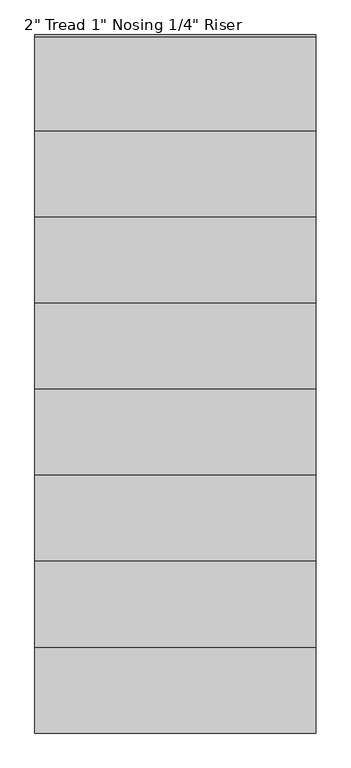
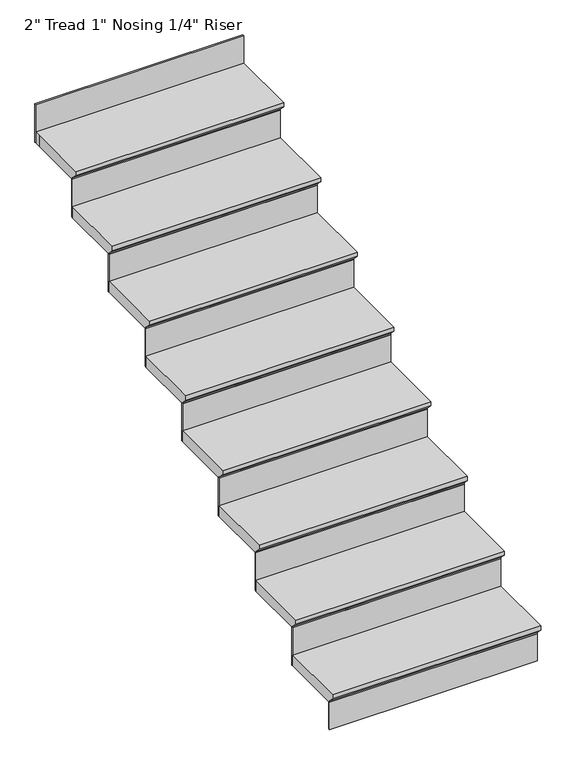
"""IFC4 building model written with IfcOpenShell, lengths in millimetres: stair flight geometry."""

from ifc_helpers import new_model, si_unit, origin, place, context, project, spatial, faceted_brep, source, transform, mapped, element, save


def stair_flight_342035e6(model_context):
    return source(origin(), model_context, "Body", "Brep", [
        faceted_brep([(-11728.968339, 6177.243496, 3968.75), (-11728.968339, 6177.243496, 3987.8), (-12643.368339, 6177.243496, 3987.8), (-12643.368339, 6177.243496, 3968.75), (-11728.968339, 6202.643496, 3943.35), (-12643.368339, 6202.643496, 3943.35), (-11728.968339, 6482.043496, 3987.8), (-12643.368339, 6482.043496, 3987.8), (-12643.368339, 6202.643496, 3937.0), (-12643.368339, 6482.043496, 3937.0), (-11728.968339, 6482.043496, 3937.0), (-11728.968339, 6202.643496, 3937.0)], [[[0, 1, 2, 3]], [[4, 0, 3, 5]], [[2, 1, 6, 7]], [[8, 9, 10, 11]], [[2, 7, 9, 8, 5, 3]], [[8, 11, 4, 5]], [[6, 1, 0, 4, 11, 10]], [[7, 6, 10, 9]]]),
        faceted_brep([(-11728.968339, 6202.643496, 3937.0), (-11728.968339, 6202.643496, 3810.0), (-11728.968339, 6208.993496, 3810.0), (-11728.968339, 6208.993496, 3937.0), (-12643.368339, 6202.643496, 3937.0), (-12643.368339, 6208.993496, 3937.0), (-12643.368339, 6208.993496, 3810.0), (-12643.368339, 6202.643496, 3810.0)], [[[0, 1, 2, 3]], [[4, 5, 6, 7]], [[1, 0, 4, 7]], [[2, 1, 7, 6]], [[3, 2, 6, 5]], [[0, 3, 5, 4]]]),
        faceted_brep([(-11728.968339, 6482.043496, 4114.8), (-11728.968339, 6482.043496, 3937.0), (-11728.968339, 6488.393496, 3937.0), (-11728.968339, 6488.393496, 4114.8), (-12643.368339, 6482.043496, 4114.8), (-12643.368339, 6488.393496, 4114.8), (-12643.368339, 6488.393496, 3937.0), (-12643.368339, 6482.043496, 3937.0)], [[[0, 1, 2, 3]], [[4, 5, 6, 7]], [[1, 0, 4, 7]], [[2, 1, 7, 6]], [[3, 2, 6, 5]], [[0, 3, 5, 4]]]),
        faceted_brep([(-12643.368339, 6456.643496, 4165.6), (-11728.968339, 6456.643496, 4165.6), (-11728.968339, 6761.443496, 4165.6), (-12643.368339, 6761.443496, 4165.6), (-12643.368339, 6482.043496, 4114.8), (-12643.368339, 6761.443496, 4114.8), (-11728.968339, 6761.443496, 4114.8), (-11728.968339, 6482.043496, 4114.8), (-12643.368339, 6482.043496, 4121.15), (-12643.368339, 6456.643496, 4146.55), (-11728.968339, 6482.043496, 4121.15), (-11728.968339, 6456.643496, 4146.55)], [[[0, 1, 2, 3]], [[4, 5, 6, 7]], [[0, 3, 5, 4, 8, 9]], [[4, 7, 10, 8]], [[2, 1, 11, 10, 7, 6]], [[3, 2, 6, 5]], [[11, 1, 0, 9]], [[10, 11, 9, 8]]]),
        faceted_brep([(-11728.968339, 6761.443496, 4292.6), (-11728.968339, 6761.443496, 4114.8), (-11728.968339, 6767.793496, 4114.8), (-11728.968339, 6767.793496, 4292.6), (-12643.368339, 6761.443496, 4292.6), (-12643.368339, 6767.793496, 4292.6), (-12643.368339, 6767.793496, 4114.8), (-12643.368339, 6761.443496, 4114.8)], [[[0, 1, 2, 3]], [[4, 5, 6, 7]], [[1, 0, 4, 7]], [[2, 1, 7, 6]], [[3, 2, 6, 5]], [[0, 3, 5, 4]]]),
        faceted_brep([(-12643.368339, 6736.043496, 4343.4), (-11728.968339, 6736.043496, 4343.4), (-11728.968339, 7040.843496, 4343.4), (-12643.368339, 7040.843496, 4343.4), (-12643.368339, 6761.443496, 4292.6), (-12643.368339, 7040.843496, 4292.6), (-11728.968339, 7040.843496, 4292.6), (-11728.968339, 6761.443496, 4292.6), (-12643.368339, 6761.443496, 4298.95), (-12643.368339, 6736.043496, 4324.35), (-11728.968339, 6761.443496, 4298.95), (-11728.968339, 6736.043496, 4324.35)], [[[0, 1, 2, 3]], [[4, 5, 6, 7]], [[0, 3, 5, 4, 8, 9]], [[4, 7, 10, 8]], [[2, 1, 11, 10, 7, 6]], [[3, 2, 6, 5]], [[11, 1, 0, 9]], [[10, 11, 9, 8]]]),
        faceted_brep([(-11728.968339, 7040.843496, 4470.4), (-11728.968339, 7040.843496, 4292.6), (-11728.968339, 7047.193496, 4292.6), (-11728.968339, 7047.193496, 4470.4), (-12643.368339, 7040.843496, 4470.4), (-12643.368339, 7047.193496, 4470.4), (-12643.368339, 7047.193496, 4292.6), (-12643.368339, 7040.843496, 4292.6)], [[[0, 1, 2, 3]], [[4, 5, 6, 7]], [[1, 0, 4, 7]], [[2, 1, 7, 6]], [[3, 2, 6, 5]], [[0, 3, 5, 4]]]),
        faceted_brep([(-12643.368339, 7015.443496, 4521.2), (-11728.968339, 7015.443496, 4521.2), (-11728.968339, 7320.243496, 4521.2), (-12643.368339, 7320.243496, 4521.2), (-12643.368339, 7040.843496, 4470.4), (-12643.368339, 7320.243496, 4470.4), (-11728.968339, 7320.243496, 4470.4), (-11728.968339, 7040.843496, 4470.4), (-12643.368339, 7040.843496, 4476.75), (-12643.368339, 7015.443496, 4502.15), (-11728.968339, 7040.843496, 4476.75), (-11728.968339, 7015.443496, 4502.15)], [[[0, 1, 2, 3]], [[4, 5, 6, 7]], [[0, 3, 5, 4, 8, 9]], [[4, 7, 10, 8]], [[2, 1, 11, 10, 7, 6]], [[3, 2, 6, 5]], [[11, 1, 0, 9]], [[10, 11, 9, 8]]]),
        faceted_brep([(-11728.968339, 7320.243496, 4648.2), (-11728.968339, 7320.243496, 4470.4), (-11728.968339, 7326.593496, 4470.4), (-11728.968339, 7326.593496, 4648.2), (-12643.368339, 7320.243496, 4648.2), (-12643.368339, 7326.593496, 4648.2), (-12643.368339, 7326.593496, 4470.4), (-12643.368339, 7320.243496, 4470.4)], [[[0, 1, 2, 3]], [[4, 5, 6, 7]], [[1, 0, 4, 7]], [[2, 1, 7, 6]], [[3, 2, 6, 5]], [[0, 3, 5, 4]]]),
        faceted_brep([(-12643.368339, 7294.843496, 4699.0), (-11728.968339, 7294.843496, 4699.0), (-11728.968339, 7599.643496, 4699.0), (-12643.368339, 7599.643496, 4699.0), (-12643.368339, 7320.243496, 4648.2), (-12643.368339, 7599.643496, 4648.2), (-11728.968339, 7599.643496, 4648.2), (-11728.968339, 7320.243496, 4648.2), (-12643.368339, 7320.243496, 4654.55), (-12643.368339, 7294.843496, 4679.95), (-11728.968339, 7320.243496, 4654.55), (-11728.968339, 7294.843496, 4679.95)], [[[0, 1, 2, 3]], [[4, 5, 6, 7]], [[0, 3, 5, 4, 8, 9]], [[4, 7, 10, 8]], [[2, 1, 11, 10, 7, 6]], [[3, 2, 6, 5]], [[11, 1, 0, 9]], [[10, 11, 9, 8]]]),
        faceted_brep([(-11728.968339, 7599.643496, 4826.0), (-11728.968339, 7599.643496, 4648.2), (-11728.968339, 7605.993496, 4648.2), (-11728.968339, 7605.993496, 4826.0), (-12643.368339, 7599.643496, 4826.0), (-12643.368339, 7605.993496, 4826.0), (-12643.368339, 7605.993496, 4648.2), (-12643.368339, 7599.643496, 4648.2)], [[[0, 1, 2, 3]], [[4, 5, 6, 7]], [[1, 0, 4, 7]], [[2, 1, 7, 6]], [[3, 2, 6, 5]], [[0, 3, 5, 4]]]),
        faceted_brep([(-12643.368339, 7574.243496, 4876.8), (-11728.968339, 7574.243496, 4876.8), (-11728.968339, 7879.043496, 4876.8), (-12643.368339, 7879.043496, 4876.8), (-12643.368339, 7599.643496, 4826.0), (-12643.368339, 7879.043496, 4826.0), (-11728.968339, 7879.043496, 4826.0), (-11728.968339, 7599.643496, 4826.0), (-12643.368339, 7599.643496, 4832.35), (-12643.368339, 7574.243496, 4857.75), (-11728.968339, 7599.643496, 4832.35), (-11728.968339, 7574.243496, 4857.75)], [[[0, 1, 2, 3]], [[4, 5, 6, 7]], [[0, 3, 5, 4, 8, 9]], [[4, 7, 10, 8]], [[2, 1, 11, 10, 7, 6]], [[3, 2, 6, 5]], [[11, 1, 0, 9]], [[10, 11, 9, 8]]]),
        faceted_brep([(-11728.968339, 7879.043496, 5003.8), (-11728.968339, 7879.043496, 4826.0), (-11728.968339, 7885.393496, 4826.0), (-11728.968339, 7885.393496, 5003.8), (-12643.368339, 7879.043496, 5003.8), (-12643.368339, 7885.393496, 5003.8), (-12643.368339, 7885.393496, 4826.0), (-12643.368339, 7879.043496, 4826.0)], [[[0, 1, 2, 3]], [[4, 5, 6, 7]], [[1, 0, 4, 7]], [[2, 1, 7, 6]], [[3, 2, 6, 5]], [[0, 3, 5, 4]]]),
        faceted_brep([(-12643.368339, 7853.643496, 5054.6), (-11728.968339, 7853.643496, 5054.6), (-11728.968339, 8158.443496, 5054.6), (-12643.368339, 8158.443496, 5054.6), (-12643.368339, 7879.043496, 5003.8), (-12643.368339, 8158.443496, 5003.8), (-11728.968339, 8158.443496, 5003.8), (-11728.968339, 7879.043496, 5003.8), (-12643.368339, 7879.043496, 5010.15), (-12643.368339, 7853.643496, 5035.55), (-11728.968339, 7879.043496, 5010.15), (-11728.968339, 7853.643496, 5035.55)], [[[0, 1, 2, 3]], [[4, 5, 6, 7]], [[0, 3, 5, 4, 8, 9]], [[4, 7, 10, 8]], [[2, 1, 11, 10, 7, 6]], [[3, 2, 6, 5]], [[11, 1, 0, 9]], [[10, 11, 9, 8]]]),
        faceted_brep([(-11728.968339, 8437.843496, 5359.4), (-11728.968339, 8437.843496, 5181.6), (-11728.968339, 8444.193496, 5181.6), (-11728.968339, 8444.193496, 5359.4), (-12643.368339, 8437.843496, 5359.4), (-12643.368339, 8444.193496, 5359.4), (-12643.368339, 8444.193496, 5181.6), (-12643.368339, 8437.843496, 5181.6)], [[[0, 1, 2, 3]], [[4, 5, 6, 7]], [[1, 0, 4, 7]], [[2, 1, 7, 6]], [[3, 2, 6, 5]], [[0, 3, 5, 4]]]),
        faceted_brep([(-11728.968339, 8158.443496, 5181.6), (-11728.968339, 8158.443496, 5003.8), (-11728.968339, 8164.793496, 5003.8), (-11728.968339, 8164.793496, 5181.6), (-12643.368339, 8158.443496, 5181.6), (-12643.368339, 8164.793496, 5181.6), (-12643.368339, 8164.793496, 5003.8), (-12643.368339, 8158.443496, 5003.8)], [[[0, 1, 2, 3]], [[4, 5, 6, 7]], [[1, 0, 4, 7]], [[2, 1, 7, 6]], [[3, 2, 6, 5]], [[0, 3, 5, 4]]]),
        faceted_brep([(-12643.368339, 8437.843496, 5232.4), (-12643.368339, 8412.443496, 5232.4), (-12643.368339, 8133.043496, 5232.4), (-11728.968339, 8133.043496, 5232.4), (-11728.968339, 8437.843496, 5232.4), (-12643.368339, 8412.443496, 5181.6), (-12643.368339, 8437.843496, 5181.6), (-11728.968339, 8437.843496, 5181.6), (-11728.968339, 8158.443496, 5181.6), (-12643.368339, 8158.443496, 5181.6), (-12643.368339, 8158.443496, 5187.95), (-12643.368339, 8133.043496, 5213.35), (-11728.968339, 8158.443496, 5187.95), (-11728.968339, 8133.043496, 5213.35)], [[[0, 1, 2, 3, 4]], [[5, 6, 7, 8, 9]], [[1, 0, 6, 5]], [[2, 1, 5, 9, 10, 11]], [[9, 8, 12, 10]], [[4, 3, 13, 12, 8, 7]], [[0, 4, 7, 6]], [[13, 3, 2, 11]], [[12, 13, 11, 10]]]),
    ])


if __name__ == "__main__":
    model = new_model("IFC4")
    model_context = context("Model", 3, world=origin())
    ifc_project = project(units=[si_unit("LENGTHUNIT", "METRE", prefix="MILLI")], contexts=[model_context])
    site = spatial("IfcSite", under=ifc_project)
    building = spatial("IfcBuilding", under=site)
    placement = place(None, origin())
    stair_flight_shape = stair_flight_342035e6(model_context)
    element("IfcStairFlight", 1, ObjectType="2\" Tread 1\" Nosing 1/4\" Riser", at=placement, inside=building, context=model_context, shape_type="MappedRepresentation", body=[
        mapped(stair_flight_shape, transform((0.0, 0.0, 0.0), x_axis=(1.0, 0.0, 0.0), y_axis=(0.0, 1.0, 0.0), z_axis=(0.0, 0.0, 1.0))),
    ])
    save(model, "model.ifc")
